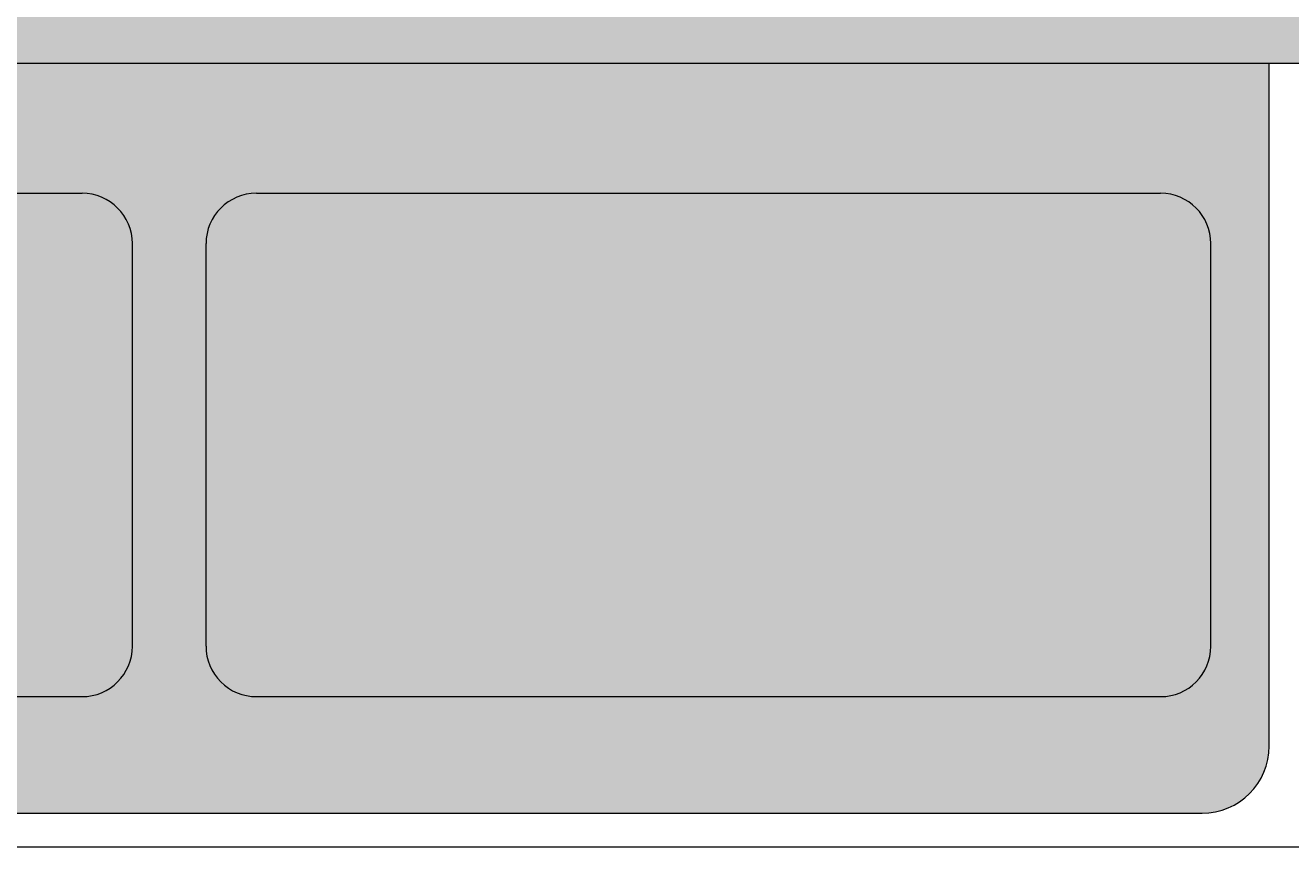
# Model space of a CAD drawing. Units: millimetres. Extents: x 27017497 to 27018854, y 7058029 to 7059154.
# Tile 24 of 91: x 27017702 to 27017732, y 7058144 to 7058163. Entities that reach past the tile are written whole.
import ezdxf

# ---------------------------------------------------------------- set-up
doc = ezdxf.new("R2010")
doc.units = ezdxf.units.MM
doc.layers.add('A-ANNO-DIMS', color=2, linetype='Continuous', lineweight=18)
doc.layers.add('A-FURN', color=8, linetype='Continuous', lineweight=18)
doc.layers.add('A-FURN-PATT', color=177, linetype='Continuous', lineweight=13, true_color=0x293189)
doc.styles.get("Standard").update_dxf_attribs({"font": 'arial.ttf'})
doc.dimstyles.get("Standard").update_dxf_attribs({"dimtxt": 0.18, "dimasz": 0.18, "dimexe": 0.18, "dimexo": 0.0625, "dimgap": 0.09, "dimtad": 0, "dimtih": 1, "dimtoh": 1, "dimdec": 4, "dimzin": 0, "dimdsep": 46, "dimtxsty": 'Standard', "dimcen": 0.09, "dimadec": 0, "dimazin": 0, "dimtfac": 1, "dimtdec": 4, "dimtofl": 0, "dimtmove": 0, "dimatfit": 3, "dimfxl": 1, "dimtolj": 1, "dimtzin": 0, "dimarcsym": 0})

# ---------------------------------------------------------------- blocks, each defined once
blk = doc.blocks.new('CAMMAT')
for p, q in [((1.27313, -0.05), (-1.27313, -0.05)), ((0.61, -0.07), (-0.61, -0.07)), ((-0.65, -0.11), (-0.65, -0.51693)), ((-0.04645, -0.1395), (-0.58524, -0.1395)), ((0.59619, -0.1395), (0.05741, -0.1395)), ((-0.61524, -0.1695), (-0.61524, -0.4095)), ((-0.01645, -0.1695), (-0.01645, -0.4095)), ((0.02741, -0.1695), (0.02741, -0.4095)), ((-0.04645, -0.4395), (-0.58524, -0.4395)), ((0.59619, -0.4395), (0.05741, -0.4395)), ((-0.6904, -0.51693), (0.68256, -0.51693))]:
    blk.add_line(p, q)
for centre, radius, start, end in [((-0.61, -0.11), 0.04, 90, 180), ((-0.58524, -0.1695), 0.03, 90, 180), ((-0.04645, -0.1695), 0.03, 360, 90), ((0.05741, -0.1695), 0.03, 90, 180), ((-0.58524, -0.4095), 0.03, 180, 270), ((-0.04645, -0.4095), 0.03, 270, 360), ((0.05741, -0.4095), 0.03, 180, 270)]:
    blk.add_arc(centre, radius, start, end)
blk = doc.blocks.new('*D47')
at = {"layer": 'A-ANNO-DIMS', "color": 0, "lineweight": -2, "transparency": 16777216}
for p, q in [((27017561.166, 7058294.35), (27017561.166, 7058028.6)), ((27018790.606, 7058294.35), (27018790.606, 7058028.6)), ((27017561.346, 7058028.78), (27018175.431, 7058028.78)), ((27018790.426, 7058028.78), (27018176.341, 7058028.78))]:
    blk.add_line(p, q, dxfattribs=at)
at = {"layer": 'A-ANNO-DIMS', "color": 0, "transparency": 16777216}
for points in [[(27017561.346, 7058028.81), (27017561.346, 7058028.75), (27017561.166, 7058028.78)], [(27018790.426, 7058028.81), (27018790.426, 7058028.75), (27018790.606, 7058028.78)]]:
    blk.add_solid(points, dxfattribs=at)
at = {"layer": 'Defpoints', "color": 0, "transparency": 16777216}
for p in [(27017561.166, 7058294.412), (27018790.606, 7058294.412), (27018790.606, 7058028.78)]:
    blk.add_point(p, dxfattribs=at)
at = {"layer": 'A-ANNO-DIMS', "color": 0, "transparency": 16777216, "insert": (27018175.886, 7058028.78), "char_height": 0.18, "attachment_point": 5}
blk.add_mtext('\\A1;1229.4', dxfattribs=at)
blk = doc.blocks.new('*D48')
at = {"layer": 'A-ANNO-DIMS', "color": 0, "lineweight": -2, "transparency": 16777216}
for p, q in [((27018463.498, 7058622.912), (27017497.536, 7058622.912)), ((27017497.716, 7058622.732), (27017497.716, 7058357.753)), ((27017497.716, 7058092.41), (27017497.716, 7058357.389)), ((27018555.129, 7058092.23), (27017497.536, 7058092.23))]:
    blk.add_line(p, q, dxfattribs=at)
at = {"layer": 'A-ANNO-DIMS', "color": 0, "transparency": 16777216}
for points in [[(27017497.686, 7058622.732), (27017497.746, 7058622.732), (27017497.716, 7058622.912)], [(27017497.686, 7058092.41), (27017497.746, 7058092.41), (27017497.716, 7058092.23)]]:
    blk.add_solid(points, dxfattribs=at)
at = {"layer": 'Defpoints', "color": 0, "transparency": 16777216}
for p in [(27018463.561, 7058622.912), (27017497.716, 7058092.23), (27018555.192, 7058092.23)]:
    blk.add_point(p, dxfattribs=at)
at = {"layer": 'A-ANNO-DIMS', "color": 0, "transparency": 16777216, "insert": (27017497.716, 7058357.571), "char_height": 0.18, "attachment_point": 5}
blk.add_mtext('\\A1;530.7', dxfattribs=at)

msp = doc.modelspace()

# ---------------------------------------------------------------- hatches: boundary and pattern name
at = {"layer": 'A-FURN-PATT'}
h = msp.add_hatch(color=256, dxfattribs=at)
h.dxf.hatch_style = 1
h.paths.add_polyline_path([(27017731.53, 7058218.852, 0.414214), (27017729.937, 7058220.445), (27017681.344, 7058220.445, 0.414214), (27017679.751, 7058218.852), (27017679.751, 7058174.658), (27017683.647, 7058174.959), (27017687.23, 7058175.46), (27017689.748, 7058176.196), (27017691.461, 7058177.277), (27017692.628, 7058178.816), (27017693.508, 7058180.922), (27017694.36, 7058183.707), (27017694.963, 7058180.902), (27017695.506, 7058178.662), (27017696.096, 7058176.759), (27017696.84, 7058174.966), (27017697.847, 7058173.059), (27017699.222, 7058170.809), (27017701.073, 7058167.99), (27017703.508, 7058164.376), (27017705.943, 7058167.99), (27017707.794, 7058170.809), (27017709.169, 7058173.059), (27017710.176, 7058174.966), (27017710.92, 7058176.759), (27017711.51, 7058178.662), (27017712.053, 7058180.902), (27017712.656, 7058183.707), (27017713.508, 7058180.922), (27017714.388, 7058178.816), (27017715.555, 7058177.277), (27017717.268, 7058176.196), (27017719.786, 7058175.46), (27017723.369, 7058174.959), (27017728.274, 7058174.58), (27017731.53, 7058174.396)])
h.paths.add_polyline_path([(27017723.369, 7058174.959), (27017719.786, 7058175.46), (27017717.268, 7058176.196), (27017715.555, 7058177.277), (27017714.388, 7058178.816), (27017713.508, 7058180.922), (27017712.656, 7058183.707), (27017712.053, 7058180.902), (27017711.51, 7058178.662), (27017710.92, 7058176.759), (27017710.176, 7058174.966), (27017709.169, 7058173.059), (27017707.794, 7058170.809), (27017705.943, 7058167.99), (27017703.508, 7058164.376), (27017734.763, 7058174.214), (27017728.274, 7058174.58)])
h.paths.add_polyline_path([(27017696.84, 7058174.966), (27017696.096, 7058176.759), (27017695.506, 7058178.662), (27017694.963, 7058180.902), (27017694.36, 7058183.707), (27017693.508, 7058180.922), (27017692.628, 7058178.816), (27017691.461, 7058177.277), (27017689.748, 7058176.196), (27017687.23, 7058175.46), (27017683.647, 7058174.959), (27017679.751, 7058174.658), (27017678.741, 7058174.58), (27017672.253, 7058174.214), (27017703.508, 7058164.376), (27017701.073, 7058167.99), (27017699.222, 7058170.809), (27017697.847, 7058173.059)])
h.paths.add_polyline_path([(27017678.454, 7058172.262), (27017678.454, 7058162.569), (27017733.139, 7058162.569), (27017733.139, 7058173.703), (27017703.508, 7058164.376)])
h.paths.add_polyline_path([(27017730.145, 7058158.291, 0.41419), (27017728.95, 7058159.485), (27017707.491, 7058159.485, 0.414214), (27017706.296, 7058158.29), (27017706.296, 7058148.731, 0.414214), (27017707.491, 7058147.536), (27017728.95, 7058147.536, 0.414237), (27017730.145, 7058148.731)], flags=0)
h.paths.add_polyline_path([(27017731.53, 7058162.569), (27017679.751, 7058162.569), (27017679.751, 7058146.361, 0.414214), (27017681.344, 7058144.768), (27017729.937, 7058144.768, 0.414214), (27017731.53, 7058146.361)])
h.paths.add_polyline_path([(27017703.354, 7058159.485, -0.41419), (27017704.549, 7058158.291), (27017704.549, 7058148.731, -0.414237), (27017703.354, 7058147.536), (27017681.894, 7058147.536, -0.41419), (27017680.699, 7058148.731), (27017680.699, 7058158.29, -0.414237), (27017681.894, 7058159.485)], flags=0)
h.paths.add_polyline_path([(27017707.491, 7058159.485), (27017728.95, 7058159.485, -0.41419), (27017730.145, 7058158.291), (27017730.145, 7058148.731, -0.414237), (27017728.95, 7058147.536), (27017707.491, 7058147.536, -0.414214), (27017706.296, 7058148.731), (27017706.296, 7058158.29, -0.414214)], flags=16)
h.paths.add_polyline_path([(27017704.549, 7058158.291, 0.41419), (27017703.354, 7058159.485), (27017681.894, 7058159.485, 0.414237), (27017680.699, 7058158.29), (27017680.699, 7058148.731, 0.41419), (27017681.894, 7058147.536), (27017703.354, 7058147.536, 0.414237), (27017704.549, 7058148.731)], flags=16)
h.paths.add_polyline_path([(27017752.64, 7058160.7), (27017732.725, 7058160.7), (27017732.725, 7058144.768), (27017752.64, 7058144.768)])
h.paths.add_polyline_path([(27017748.698, 7058152.101, -1), (27017736.749, 7058152.101, -1)], flags=16)
h.paths.add_polyline_path([(27017746.424, 7058152.101, -1), (27017739.024, 7058152.101, -1)], flags=0)
h.paths.add_polyline_path([(27017678.556, 7058160.7), (27017658.641, 7058160.7), (27017658.641, 7058144.768), (27017678.556, 7058144.768)])
h.paths.add_polyline_path([(27017674.806, 7058152.101, -1), (27017662.857, 7058152.101, -1)], flags=16)
h.paths.add_polyline_path([(27017672.531, 7058152.101, -1), (27017665.131, 7058152.101, -1)], flags=0)
h = msp.add_hatch(color=256, dxfattribs=at)
h.dxf.hatch_style = 1
h.paths.add_polyline_path([(27017730.145, 7058158.291, 0.41419), (27017728.95, 7058159.485), (27017707.491, 7058159.485, 0.414214), (27017706.296, 7058158.29), (27017706.296, 7058148.731, 0.414214), (27017707.491, 7058147.536), (27017728.95, 7058147.536, 0.414237), (27017730.145, 7058148.731)])
h.paths.add_polyline_path([(27017704.549, 7058158.291, 0.41419), (27017703.354, 7058159.485), (27017681.894, 7058159.485, 0.414237), (27017680.699, 7058158.29), (27017680.699, 7058148.731, 0.41419), (27017681.894, 7058147.536), (27017703.354, 7058147.536, 0.414237), (27017704.549, 7058148.731)])

# ---------------------------------------------------------------- block references
at = {"layer": 'A-FURN', "xscale": 39.82996475819422, "yscale": 39.82996475819422, "zscale": 39.82996475819422, "rotation": 180}
msp.add_blockref('CAMMAT', (27017705.64, 7058141.98), dxfattribs=at)

# ---------------------------------------------------------------- dimensions: what is measured, and where the dimension line sits
at = {"layer": 'A-ANNO-DIMS'}
dim = msp.add_linear_dim(base=(27017497.716, 7058092.23), p1=(27018463.561, 7058622.912), p2=(27018555.192, 7058092.23), angle=90, dimstyle='Standard', override={"dimdec": 1, "dimlfac": 1, "dimrnd": 0, "dimzin": 0, "dimdsep": 46, "dimlunit": 2}, dxfattribs=at)
dim.commit()
dim.dimension.update_dxf_attribs({"geometry": '*D48', "text_midpoint": (27017497.716, 7058357.571)})
dim = msp.add_linear_dim(base=(27018790.606, 7058028.78), p1=(27017561.166, 7058294.412), p2=(27018790.606, 7058294.412), dimstyle='Standard', override={"dimdec": 1, "dimlfac": 1, "dimrnd": 0, "dimzin": 0, "dimdsep": 46, "dimlunit": 2}, dxfattribs=at)
dim.commit()
dim.dimension.update_dxf_attribs({"geometry": '*D47', "text_midpoint": (27018175.886, 7058028.78)})

doc.saveas('drawing.dxf')
